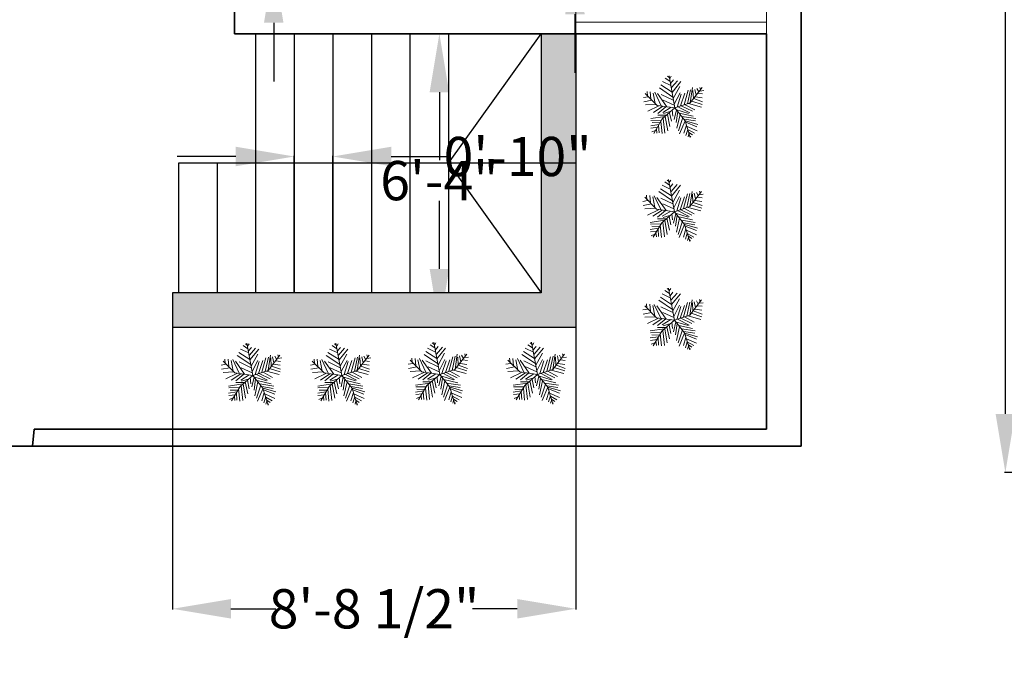
# Model space of a CAD drawing. Units: inches. Extents: x 19 to 15718, y 7 to 930.
# Tile 3 of 11: x 14988 to 15243, y 300 to 468. Entities that reach past the tile are written whole.
import ezdxf

# ---------------------------------------------------------------- set-up
doc = ezdxf.new("R2010")
doc.units = ezdxf.units.IN
doc.header["$MEASUREMENT"] = 0
for name, color, linetype, lineweight in [('A-ANNO-DIMS', 2, 'Continuous', 18), ('A-FLOR-STRS', 7, 'Continuous', 25), ('A-GLAZ', 4, 'Continuous', 18), ('A-WALL', 7, 'Continuous', 35), ('L-PLNT', 3, 'Continuous', 13)]:
    doc.layers.add(name, color=color, linetype=linetype, lineweight=lineweight)
doc.layers.add('A-WALL-PATT', color=18, linetype='Continuous', lineweight=13, true_color=0x000000)
doc.styles.get("Standard").update_dxf_attribs({"font": 'arial.ttf'})
doc.dimstyles.get("Standard").update_dxf_attribs({"dimtxt": 10.18, "dimasz": 15.18, "dimexe": 0.18, "dimexo": 0.0625, "dimgap": 0.09, "dimtad": 0, "dimtih": 1, "dimtoh": 1, "dimdec": 0, "dimzin": 0, "dimdsep": 46, "dimlunit": 3, "dimtxsty": 'Standard', "dimcen": 0.09, "dimadec": 0, "dimazin": 0, "dimtfac": 1, "dimtdec": 0, "dimtofl": 0, "dimtmove": 0, "dimatfit": 3, "dimfxl": 1, "dimtolj": 1, "dimtzin": 0, "dimarcsym": 0})

# ---------------------------------------------------------------- blocks, each defined once
blk = doc.blocks.new('*U13')
for p, q in [((-8.737, 47.138), (-17.069, 52.711)), ((-10.186, 53.64), (-13.084, 55.962)), ((0, 0), (-10.5, 57)), ((-9.099, 51.782), (-6.563, 55.962)), ((-3.665, 19.273), (-27.574, 35.527)), ((-5.114, 28.097), (-24.676, 40.636)), ((-7.288, 39.707), (-21.778, 46.673)), ((-7.65, 43.423), (-2.578, 49.46)), ((-5.839, 35.992), (4.667, 48.067)), ((-5.114, 27.632), (10.463, 46.673)), ((-2.941, 16.486), (8.652, 37.85)), ((27, 9), (48, 36)), ((27.127, 9.056), (31.112, 35.992)), ((44.153, 36.456), (45.239, 32.741)), ((-47.498, 19.737), (-55.83, 18.344)), ((-31.5, 4.5), (-52.5, 25.5)), ((-48.585, 21.131), (-49.309, 29.026)), ((-43.513, 28.561), (-42.427, 15.558)), ((-38.442, 26.239), (-34.819, 7.663)), ((-35.544, 28.097), (-24.314, 3.947)), ((-14.533, 2.09), (-30.834, 25.31)), ((-24.314, 23.917), (-2.941, 13.7)), ((-1.129, 6.734), (9.014, 26.704)), ((3.942, 1.625), (11.187, 24.381)), ((10.101, 3.483), (17.708, 26.239)), ((16.259, 5.805), (23.142, 31.348)), ((22.055, 7.198), (27.489, 32.277)), ((31.836, 30.883), (32.561, 16.486)), ((35.096, 32.741), (37.27, 22.524)), ((36.183, 19.737), (48.137, 17.88)), ((38.719, 34.134), (41.979, 28.561)), ((40.53, 25.775), (48.862, 24.846)), ((43.791, 29.954), (51.036, 30.883)), ((-40.615, 13.7), (-55.105, 10.913)), ((-33.37, 6.269), (-52.207, 5.34)), ((-28.299, 3.483), (-47.86, -5.805)), ((-21.416, 3.018), (-38.079, -8.128)), ((0, 0), (-31.5, 4.5)), ((-15.982, 2.09), (-30.11, -9.521)), ((0, 0), (-22.5, -19.5)), ((-6.563, 1.161), (-21.416, -8.128)), ((-20.691, 13.7), (-1.129, 4.876)), ((0, 0), (27, 9)), ((0, 0), (18, -22.5)), ((6.478, 1.625), (26.04, -8.592)), ((11.187, 3.483), (30.749, -5.805)), ((18.07, 5.805), (35.096, -3.483)), ((24.229, 7.663), (46.688, 1.625)), ((29.662, 12.307), (48.137, 6.269)), ((33.285, 16.486), (48.862, 10.913)), ((-17.431, -15.094), (-42.789, -18.809)), ((-15.257, -12.772), (-30.11, -12.772)), ((-6.563, -5.805), (-19.967, -9.985)), ((-17.069, -15.094), (-12.721, -40.172)), ((-13.446, -11.378), (-8.737, -32.741)), ((-9.461, -8.592), (-6.201, -23.453)), ((-4.752, -3.483), (-3.665, -14.629)), ((2.493, -3.019), (-1.491, -20.202)), ((1.769, -2.555), (24.229, -9.521)), ((5.029, -6.27), (2.131, -25.775)), ((9.014, -11.378), (3.58, -35.992)), ((14.085, -16.951), (6.478, -40.172)), ((7.565, -9.056), (32.198, -14.629)), ((12.274, -15.094), (36.907, -18.809)), ((-28.299, -29.026), (-42.789, -31.348)), ((-24.314, -21.596), (-42.427, -22.06)), ((-30.834, -34.135), (-42.427, -35.528)), ((-26.849, -26.24), (-40.253, -25.775)), ((-22.5, -19.5), (-37.5, -45)), ((-29.023, -30.884), (-27.936, -43.887)), ((-25.038, -23.918), (-22.865, -45.281)), ((-20.691, -18.345), (-17.793, -44.352)), ((18.07, -22.524), (8.289, -45.745)), ((20.244, -30.419), (15.897, -44.816)), ((16.259, -19.738), (36.183, -22.989)), ((18, -22.5), (27, -52.5)), ((18.433, -22.524), (40.53, -29.026)), ((19.157, -25.311), (38.719, -33.206)), ((21.331, -32.741), (39.081, -40.636)), ((-34.457, -39.708), (-40.978, -42.494)), ((-32.646, -36.921), (-31.921, -44.352)), ((22.78, -37.85), (19.519, -48.532)), ((22.78, -38.314), (34.372, -44.816)), ((24.591, -45.745), (23.142, -50.854)), ((24.591, -43.423), (30.749, -47.603)), ((26.764, -49.925), (28.213, -50.854))]:
    blk.add_line(p, q)
blk = doc.blocks.new('*D17')
at = {"layer": 'A-ANNO-DIMS', "color": 0, "lineweight": -2, "transparency": 16777216}
for p, q in [((15266.62, 830.27), (15243.58, 830.27)), ((15243.76, 815.09), (15243.76, 595.52)), ((15243.76, 365.38), (15243.76, 584.95)), ((15266.62, 350.2), (15243.58, 350.2))]:
    blk.add_line(p, q, dxfattribs=at)
at = {"layer": 'A-ANNO-DIMS', "color": 0, "transparency": 16777216}
for points in [[(15241.23, 815.09), (15246.29, 815.09), (15243.76, 830.27)], [(15241.23, 365.38), (15246.29, 365.38), (15243.76, 350.2)]]:
    blk.add_solid(points, dxfattribs=at)
at = {"layer": 'Defpoints', "color": 0, "transparency": 16777216}
for p in [(15266.68, 830.27), (15243.76, 350.2), (15266.68, 350.2)]:
    blk.add_point(p, dxfattribs=at)
at = {"layer": 'A-ANNO-DIMS', "color": 0, "transparency": 16777216, "insert": (15243.76, 590.24), "char_height": 10.18, "attachment_point": 5}
blk.add_mtext("\\A1;40'", dxfattribs=at)
blk = doc.blocks.new('*D36')
at = {"layer": 'A-ANNO-DIMS', "color": 0, "lineweight": -2, "transparency": 16777216}
for p, q in [((15054.04, 525.18), (15054.04, 540.36)), ((15049.9, 510), (15054.22, 510)), ((15049.9, 482), (15054.22, 482)), ((15054.04, 466.82), (15054.04, 451.64))]:
    blk.add_line(p, q, dxfattribs=at)
at = {"layer": 'A-ANNO-DIMS', "color": 0, "transparency": 16777216}
for points in [[(15051.51, 525.18), (15056.57, 525.18), (15054.04, 510)], [(15051.51, 466.82), (15056.57, 466.82), (15054.04, 482)]]:
    blk.add_solid(points, dxfattribs=at)
at = {"layer": 'Defpoints', "color": 0, "transparency": 16777216}
for p in [(15049.84, 510), (15054.04, 510), (15049.84, 482)]:
    blk.add_point(p, dxfattribs=at)
at = {"layer": 'A-ANNO-DIMS', "color": 0, "transparency": 16777216, "insert": (15054.04, 496), "char_height": 10.18, "attachment_point": 5}
blk.add_mtext('\\A1;WINDOW FRAME 2\'-4" TYP.', dxfattribs=at)
blk = doc.blocks.new('*D37')
at = {"layer": 'A-ANNO-DIMS', "color": 0, "lineweight": -2, "transparency": 16777216}
for p, q in [((15043.84, 481.93), (15043.84, 477.62)), ((15049.84, 481.93), (15049.84, 477.62)), ((15028.66, 477.8), (15013.48, 477.8)), ((15065.02, 477.8), (15080.2, 477.8))]:
    blk.add_line(p, q, dxfattribs=at)
at = {"layer": 'A-ANNO-DIMS', "color": 0, "transparency": 16777216}
for points in [[(15028.66, 480.33), (15028.66, 475.27), (15043.84, 477.8)], [(15065.02, 480.33), (15065.02, 475.27), (15049.84, 477.8)]]:
    blk.add_solid(points, dxfattribs=at)
at = {"layer": 'Defpoints', "color": 0, "transparency": 16777216}
for p in [(15043.84, 482), (15049.84, 482), (15049.84, 477.8)]:
    blk.add_point(p, dxfattribs=at)
at = {"layer": 'A-ANNO-DIMS', "color": 0, "transparency": 16777216, "insert": (15111.31, 477.8), "char_height": 10.18, "attachment_point": 5}
blk.add_mtext('\\A1;0\'-6" TYP.', dxfattribs=at)
blk = doc.blocks.new('*D60')
at = {"layer": 'A-ANNO-DIMS', "color": 0, "lineweight": -2, "transparency": 16777216}
for p, q in [((15110.6, 483.39), (15095.42, 483.39)), ((15125.78, 484.16), (15125.78, 483.21)), ((15131.32, 484.16), (15131.32, 483.21)), ((15146.5, 483.39), (15161.68, 483.39))]:
    blk.add_line(p, q, dxfattribs=at)
at = {"layer": 'A-ANNO-DIMS', "color": 0, "transparency": 16777216}
for points in [[(15110.6, 485.92), (15110.6, 480.86), (15125.78, 483.39)], [(15146.5, 485.92), (15146.5, 480.86), (15131.32, 483.39)]]:
    blk.add_solid(points, dxfattribs=at)
at = {"layer": 'Defpoints', "color": 0, "transparency": 16777216}
for p in [(15125.78, 484.23), (15131.32, 484.23), (15131.32, 483.39)]:
    blk.add_point(p, dxfattribs=at)
at = {"layer": 'A-ANNO-DIMS', "color": 0, "transparency": 16777216, "insert": (15253.56, 483.39), "char_height": 10.18, "attachment_point": 5}
blk.add_mtext('\\A1;GAS BURNER 0\'-5 1/2" TYP.', dxfattribs=at)
blk = doc.blocks.new('*D61')
at = {"layer": 'A-ANNO-DIMS', "color": 0, "lineweight": -2, "transparency": 16777216}
for p, q in [((15132.15, 504.55), (15132.15, 519.73)), ((15132.15, 519.73), (15147.33, 519.73)), ((15131.38, 489.37), (15132.33, 489.37)), ((15131.38, 484.23), (15132.33, 484.23)), ((15132.15, 469.05), (15132.15, 453.87))]:
    blk.add_line(p, q, dxfattribs=at)
at = {"layer": 'A-ANNO-DIMS', "color": 0, "transparency": 16777216}
for points in [[(15129.62, 504.55), (15134.68, 504.55), (15132.15, 489.37)], [(15129.62, 469.05), (15134.68, 469.05), (15132.15, 484.23)]]:
    blk.add_solid(points, dxfattribs=at)
at = {"layer": 'Defpoints', "color": 0, "transparency": 16777216}
for p in [(15131.32, 489.37), (15132.15, 489.37), (15131.32, 484.23)]:
    blk.add_point(p, dxfattribs=at)
at = {"layer": 'A-ANNO-DIMS', "color": 0, "transparency": 16777216, "insert": (15178.44, 519.73), "char_height": 10.18, "attachment_point": 5}
blk.add_mtext('\\A1;0\'-5" TYP.', dxfattribs=at)
blk = doc.blocks.new('*D74')
at = {"layer": 'A-ANNO-DIMS', "color": 0, "lineweight": -2, "transparency": 16777216}
for p, q in [((15027.77, 387.74), (15027.77, 314.67)), ((15132.35, 387.74), (15132.35, 314.67)), ((15042.95, 314.85), (15054.57, 314.85)), ((15117.17, 314.85), (15105.55, 314.85))]:
    blk.add_line(p, q, dxfattribs=at)
at = {"layer": 'A-ANNO-DIMS', "color": 0, "transparency": 16777216}
for points in [[(15042.95, 317.38), (15042.95, 312.32), (15027.77, 314.85)], [(15117.17, 317.38), (15117.17, 312.32), (15132.35, 314.85)]]:
    blk.add_solid(points, dxfattribs=at)
at = {"layer": 'Defpoints', "color": 0, "transparency": 16777216}
for p in [(15027.77, 387.8), (15132.35, 387.8), (15132.35, 314.85)]:
    blk.add_point(p, dxfattribs=at)
at = {"layer": 'A-ANNO-DIMS', "color": 0, "transparency": 16777216, "insert": (15080.06, 314.85), "char_height": 10.18, "attachment_point": 5}
blk.add_mtext('\\A1;8\'-8 1/2"', dxfattribs=at)
blk = doc.blocks.new('*D75')
at = {"layer": 'A-ANNO-DIMS', "color": 0, "lineweight": -2, "transparency": 16777216}
for p, q in [((15132.28538, 463.995573), (15096.81788, 463.995573)), ((15096.99788, 448.815573), (15096.99788, 431.186197)), ((15096.99788, 402.981555), (15096.99788, 420.610931)), ((15132.28538, 387.801555), (15096.81788, 387.801555))]:
    blk.add_line(p, q, dxfattribs=at)
at = {"layer": 'A-ANNO-DIMS', "color": 0, "transparency": 16777216}
for points in [[(15094.46788, 448.815573), (15099.52788, 448.815573), (15096.99788, 463.995573)], [(15094.46788, 402.981555), (15099.52788, 402.981555), (15096.99788, 387.801555)]]:
    blk.add_solid(points, dxfattribs=at)
at = {"layer": 'Defpoints', "color": 0, "transparency": 16777216}
for p in [(15096.99788, 463.995573), (15132.34788, 463.995573), (15132.34788, 387.801555)]:
    blk.add_point(p, dxfattribs=at)
at = {"layer": 'A-ANNO-DIMS', "color": 0, "transparency": 16777216, "insert": (15096.99788, 425.898564), "char_height": 10.18, "attachment_point": 5}
blk.add_mtext('\\A1;6\'-4"', dxfattribs=at)
blk = doc.blocks.new('*D80')
at = {"layer": 'A-ANNO-DIMS', "color": 0, "lineweight": -2, "transparency": 16777216}
for p, q in [((15602.030581, 511.142303), (15602.030581, 526.322303)), ((15181.899116, 495.962303), (15602.210581, 495.962303)), ((15181.899116, 469.995573), (15602.210581, 469.995573)), ((15602.030581, 454.815573), (15602.030581, 439.635573))]:
    blk.add_line(p, q, dxfattribs=at)
at = {"layer": 'A-ANNO-DIMS', "color": 0, "transparency": 16777216}
for points in [[(15599.500581, 511.142303), (15604.560581, 511.142303), (15602.030581, 495.962303)], [(15599.500581, 454.815573), (15604.560581, 454.815573), (15602.030581, 469.995573)]]:
    blk.add_solid(points, dxfattribs=at)
at = {"layer": 'Defpoints', "color": 0, "transparency": 16777216}
for p in [(15181.836616, 495.962303), (15602.030581, 495.962303), (15181.836616, 469.995573)]:
    blk.add_point(p, dxfattribs=at)
at = {"layer": 'A-ANNO-DIMS', "color": 0, "transparency": 16777216, "insert": (15602.030581, 482.978938), "char_height": 10.18, "attachment_point": 5}
blk.add_mtext('\\A1;2\'-2"', dxfattribs=at)
blk = doc.blocks.new('*D86')
at = {"layer": 'A-ANNO-DIMS', "color": 0, "lineweight": -2, "transparency": 16777216}
for p, q in [((15044.17, 432.15), (15028.99, 432.15)), ((15059.35, 396.86), (15059.35, 432.33)), ((15069.35, 396.86), (15069.35, 432.33)), ((15084.53, 432.15), (15099.71, 432.15))]:
    blk.add_line(p, q, dxfattribs=at)
at = {"layer": 'A-ANNO-DIMS', "color": 0, "transparency": 16777216}
for points in [[(15044.17, 434.68), (15044.17, 429.62), (15059.35, 432.15)], [(15084.53, 434.68), (15084.53, 429.62), (15069.35, 432.15)]]:
    blk.add_solid(points, dxfattribs=at)
at = {"layer": 'Defpoints', "color": 0, "transparency": 16777216}
for p in [(15069.35, 432.15), (15059.35, 396.8), (15069.35, 396.8)]:
    blk.add_point(p, dxfattribs=at)
at = {"layer": 'A-ANNO-DIMS', "color": 0, "transparency": 16777216, "insert": (15117.28, 432.15), "char_height": 10.18, "attachment_point": 5}
blk.add_mtext('\\A1;0\'-10"', dxfattribs=at)

msp = doc.modelspace()

# ---------------------------------------------------------------- hatches: boundary and pattern name
at = {"layer": 'A-WALL-PATT'}
h = msp.add_hatch(color=256, dxfattribs=at)
h.dxf.hatch_style = 1
h.paths.add_polyline_path([(15190.84, 837), (14890.84, 837), (14890.84, 357), (14899.84, 357), (14899.84, 366), (14899.84, 528), (14904.84, 528), (14904.84, 534), (14899.84, 534), (14899.84, 698), (15004.84, 698), (15004.84, 701, -0.014283), (15004.84, 703), (15004.84, 704), (14899.84, 704), (14899.84, 828), (14987.26, 828), (15043.84, 828), (15049.84, 828), (15075.84, 828), (15081.84, 828), (15181.84, 828), (15181.84, 780), (15114.84, 780), (15114.84, 779, -0.017236), (15114.84, 777), (15114.84, 774), (15181.84, 774), (15181.84, 654), (15181.84, 648), (15181.84, 596), (15190.84, 596)])
h.paths.add_polyline_path([(15190.84, 590), (15181.84, 590), (15181.84, 470), (15181.84, 464), (15181.84, 361.43), (14991.9, 361.43), (14991.5, 357), (15190.84, 357)], flags=0)
h.paths.add_polyline_path([(15152.29, 608), (15146.29, 608), (15146.29, 596), (15049.84, 596), (15049.84, 590), (15152.29, 590)], flags=17)
h.paths.add_polyline_path([(15049.84, 615), (15048.84, 615, -0.017236), (15046.84, 615), (15043.84, 615), (15043.84, 596), (15049.84, 596)], flags=17)
edge = h.paths.add_edge_path(flags=17)
edge.add_line((15152.29, 654), (15049.84, 654))
edge.add_line((15049.84, 654), (15043.84, 654))
edge.add_line((15043.84, 654), (15043.84, 648))
edge.add_line((15043.84, 648), (15049.84, 648))
edge.add_line((15049.84, 648), (15075.84, 648))
edge.add_line((15075.84, 648), (15081.84, 648))
edge.add_line((15081.84, 648), (15117.26, 648))
edge.add_spline(control_points=[(15117.26, 648), (15117.59, 648.02), (15117.94, 648.03), (15118.71, 648.04), (15119.15, 648.02), (15119.59, 648)], knot_values=[1.499122, 1.499122, 1.499122, 1.499122, 1.618335, 1.618335, 1.770388, 1.770388, 1.770388, 1.770388], degree=3, periodic=0)
edge.add_spline(control_points=[(15127.99, 642.93), (15128, 643.28), (15127.95, 643.62), (15127.73, 644.26), (15127.57, 644.57), (15127.16, 645.13), (15126.92, 645.39), (15126.04, 646.16), (15125.28, 646.6), (15123.53, 647.31), (15122.55, 647.59), (15120.88, 647.88), (15120.24, 647.95), (15119.59, 648)], knot_values=[0, 0, 0, 0, 0.172075, 0.172075, 0.344149, 0.344149, 0.516224, 0.516224, 0.894541, 0.894541, 1.272858, 1.272858, 1.499122, 1.499122, 1.499122, 1.499122], degree=3, periodic=0)
edge.add_line((15119.59, 648), (15146.29, 648))
edge.add_line((15146.29, 648), (15146.29, 636))
edge.add_line((15146.29, 636), (15152.29, 636))
edge.add_line((15152.29, 636), (15152.29, 654))
h.paths.add_polyline_path([(15132.35, 430.4), (15123.35, 430.4), (15123.35, 396.8), (15027.77, 396.8), (15027.77, 387.8), (15132.35, 387.8)], flags=17)
h.paths.add_polyline_path([(15132.35, 464), (15123.35, 464), (15123.35, 430.4), (15132.35, 430.4)], flags=17)
h.paths.add_polyline_path([(15275.68, 583.59), (15276.07, 583.2), (15276.65, 583.2), (15280.6, 587.16), (15278.55, 589.2), (15275.68, 589.2), (15275.68, 601.2), (15266.68, 601.2), (15266.68, 350.2), (15275.68, 350.2), (15275.68, 359.2), (15275.68, 457.2), (15413.68, 457.2), (15413.68, 471.04), (15407.68, 471.04), (15407.68, 463.2), (15275.68, 463.2)])

# ---------------------------------------------------------------- linework, layer by layer
at = {"layer": 'A-FLOR-STRS'}
for p, q in [((15049.35, 464), (15049.35, 396.8)), ((15049.35, 464), (15049.35, 396.8)), ((15059.35, 464), (15059.35, 396.8)), ((15069.35, 464), (15069.35, 396.8)), ((15079.35, 464), (15079.35, 396.8)), ((15079.35, 464), (15079.35, 396.8)), ((15089.35, 464), (15089.35, 396.8)), ((15099.35, 464), (15099.35, 396.8)), ((15099.35, 430.4), (15123.35, 464)), ((15123.35, 464), (15123.35, 396.8)), ((15132.35, 464), (15132.35, 387.8)), ((15029.35, 430.4), (15029.35, 396.8)), ((15132.35, 430.4), (15029.35, 430.4)), ((15039.35, 430.4), (15039.35, 396.8)), ((15099.35, 430.4), (15123.35, 396.8)), ((15123.35, 396.8), (15027.77, 396.8)), ((15027.77, 396.8), (15027.77, 387.8)), ((15132.35, 387.8), (15027.77, 387.8))]:
    msp.add_line(p, q, dxfattribs=at)
at = {"layer": 'A-GLAZ'}
for p, q in [((15132.35, 464), (15132.35, 470)), ((15181.84, 470), (15181.84, 464)), ((15132.35, 467), (15181.84, 467))]:
    msp.add_line(p, q, dxfattribs=at)
at = {"layer": 'A-WALL'}
for p, q in [((15190.84, 837), (15190.84, 357)), ((15043.84, 464), (15043.84, 528)), ((15049.84, 464), (15043.84, 464)), ((15049.84, 464), (15181.84, 464)), ((15181.84, 464), (15181.84, 361.43)), ((14991.5, 357), (14991.9, 361.43)), ((14991.9, 361.43), (15181.84, 361.43)), ((15190.84, 357), (14890.84, 357))]:
    msp.add_line(p, q, dxfattribs=at)

# ---------------------------------------------------------------- block references
at = {"layer": 'L-PLNT', "xscale": 0.1466943770709678, "yscale": 0.1466943770709678, "zscale": 0.1466943770709678}
for p in [(15158.08, 444.74), (15157.95, 417.83), (15157.95, 389.68), (15048.61, 375.37), (15071.72, 375.37), (15097.08, 375.61), (15122.44, 375.61)]:
    msp.add_blockref('*U13', p, dxfattribs=at)

# ---------------------------------------------------------------- dimensions: what is measured, and where the dimension line sits
at = {"layer": 'A-ANNO-DIMS'}
for base, p1, p2, override, picture, middle in [((15243.76, 350.2), (15266.68, 830.27), (15266.68, 350.2), {"dimclrd": 0, "dimclre": 0, "dimclrt": 0}, '*D17', (15243.76, 590.24)), ((15602.03, 495.96), (15181.84, 470), (15181.84, 495.96), {"dimdec": 1, "dimlfac": 1, "dimrnd": 0, "dimzin": 1, "dimdsep": 46, "dimlunit": 4, "dimfrac": 2}, '*D80', (15602.03, 482.98)), ((15097, 464), (15132.35, 387.8), (15132.35, 464), {"dimdec": 1, "dimlfac": 1, "dimrnd": 0, "dimzin": 1, "dimdsep": 46, "dimlunit": 4, "dimfrac": 2}, '*D75', (15097, 425.9))]:
    dim = msp.add_linear_dim(base=base, p1=p1, p2=p2, angle=90, dimstyle='Standard', override=override, dxfattribs=at)
    dim.commit()
    dim.dimension.update_dxf_attribs({"geometry": picture, "text_midpoint": middle})
for base, p1, p2, text, picture, middle in [((15054.04, 510), (15049.84, 482), (15049.84, 510), 'WINDOW FRAME <> TYP.', '*D36', (15054.04, 496)), ((15132.15, 489.37), (15131.32, 484.23), (15131.32, 489.37), '<> TYP.', '*D61', (15178.44, 519.73))]:
    dim = msp.add_linear_dim(base=base, p1=p1, p2=p2, angle=90, text=text, dimstyle='Standard', override={"dimdec": 1, "dimlfac": 1, "dimrnd": 0, "dimzin": 1, "dimdsep": 46, "dimlunit": 4, "dimfrac": 2}, dxfattribs=at)
    dim.commit()
    dim.dimension.update_dxf_attribs({"geometry": picture, "text_midpoint": middle})
for base, p1, p2, text, picture, middle in [((15131.32, 483.39), (15125.78, 484.23), (15131.32, 484.23), 'GAS BURNER <> TYP.', '*D60', (15253.56, 483.39)), ((15049.84, 477.8), (15043.84, 482), (15049.84, 482), '<> TYP.', '*D37', (15111.31, 477.8))]:
    dim = msp.add_linear_dim(base=base, p1=p1, p2=p2, text=text, dimstyle='Standard', override={"dimdec": 1, "dimlfac": 1, "dimrnd": 0, "dimzin": 1, "dimdsep": 46, "dimlunit": 4, "dimfrac": 2}, dxfattribs=at)
    dim.commit()
    dim.dimension.update_dxf_attribs({"geometry": picture, "text_midpoint": middle})
for base, p1, p2, picture, middle in [((15069.35, 432.15), (15059.35, 396.8), (15069.35, 396.8), '*D86', (15117.28, 432.15)), ((15132.35, 314.85), (15027.77, 387.8), (15132.35, 387.8), '*D74', (15080.06, 314.85))]:
    dim = msp.add_linear_dim(base=base, p1=p1, p2=p2, dimstyle='Standard', override={"dimdec": 1, "dimlfac": 1, "dimrnd": 0, "dimzin": 1, "dimdsep": 46, "dimlunit": 4, "dimfrac": 2}, dxfattribs=at)
    dim.commit()
    dim.dimension.update_dxf_attribs({"geometry": picture, "text_midpoint": middle})

doc.saveas('drawing.dxf')
